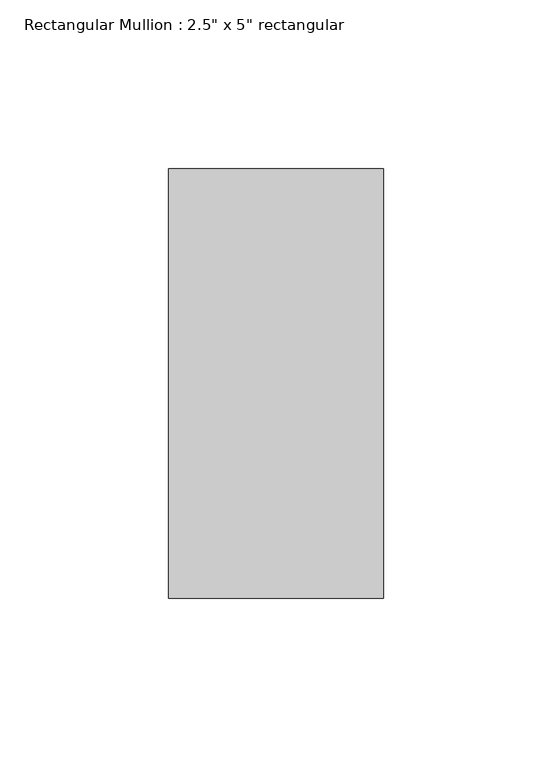
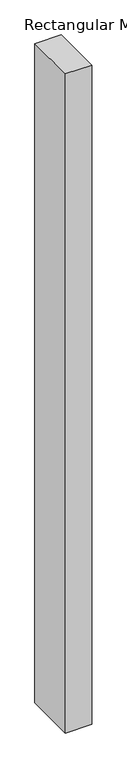
"""IFC4 building model written with IfcOpenShell, lengths in millimetres: member geometry."""

from ifc_helpers import new_model, si_unit, frame, origin, place, context, project, spatial, polyline, outline, extrude, source, transform, mapped, element, save


def member_c78c2eae(model_context):
    return source(origin(), model_context, "Body", "SweptSolid", [
        extrude(outline(polyline([(31.75, 63.5), (31.75, -63.5), (-31.75, -63.5), (-31.75, 63.5), (31.75, 63.5)])), frame((0.0, 0.0, -1676.3357893), z_axis=(0.0, 0.0, 1.0), x_axis=(1.0, 0.0, 0.0)), (0.0, 0.0, 1.0), 1676.3357893),
    ])


if __name__ == "__main__":
    model = new_model("IFC4")
    model_context = context("Model", 3, world=origin())
    ifc_project = project(units=[si_unit("LENGTHUNIT", "METRE", prefix="MILLI")], contexts=[model_context])
    site = spatial("IfcSite", under=ifc_project)
    building = spatial("IfcBuilding", under=site)
    placement = place(None, origin())
    member_shape = member_c78c2eae(model_context)
    element("IfcMember", 1, ObjectType="Rectangular Mullion : 2.5\" x 5\" rectangular", at=placement, inside=building, context=model_context, shape_type="MappedRepresentation", body=[
        mapped(member_shape, transform((0.0, 0.0, 0.0), x_axis=(1.0, 0.0, 0.0), y_axis=(0.0, 1.0, 0.0), z_axis=(0.0, 0.0, 1.0))),
    ])
    save(model, "model.ifc")

# Revit data of these elements
# Type "Rectangular Mullion : 2.5\" x 5\" rectangular"
#   built-in parameter 1007304 = 0.416667 (stored number, unit not read)
#   built-in parameter 1007301 = 0.104167 (stored number, unit not read)
#   built-in parameter 1007300 = 0.104167 (stored number, unit not read)
# Element 1 (IfcMember, "Rectangular Mullion : 2.5\" x 5\" rectangular")
#   Materials on its faces: "Aluminum"
# Materials
#   "Aluminum": class "Metal", colour RGB 247 247 247, transparency 0, Description = "Aluminum 6061", Cost = 0
